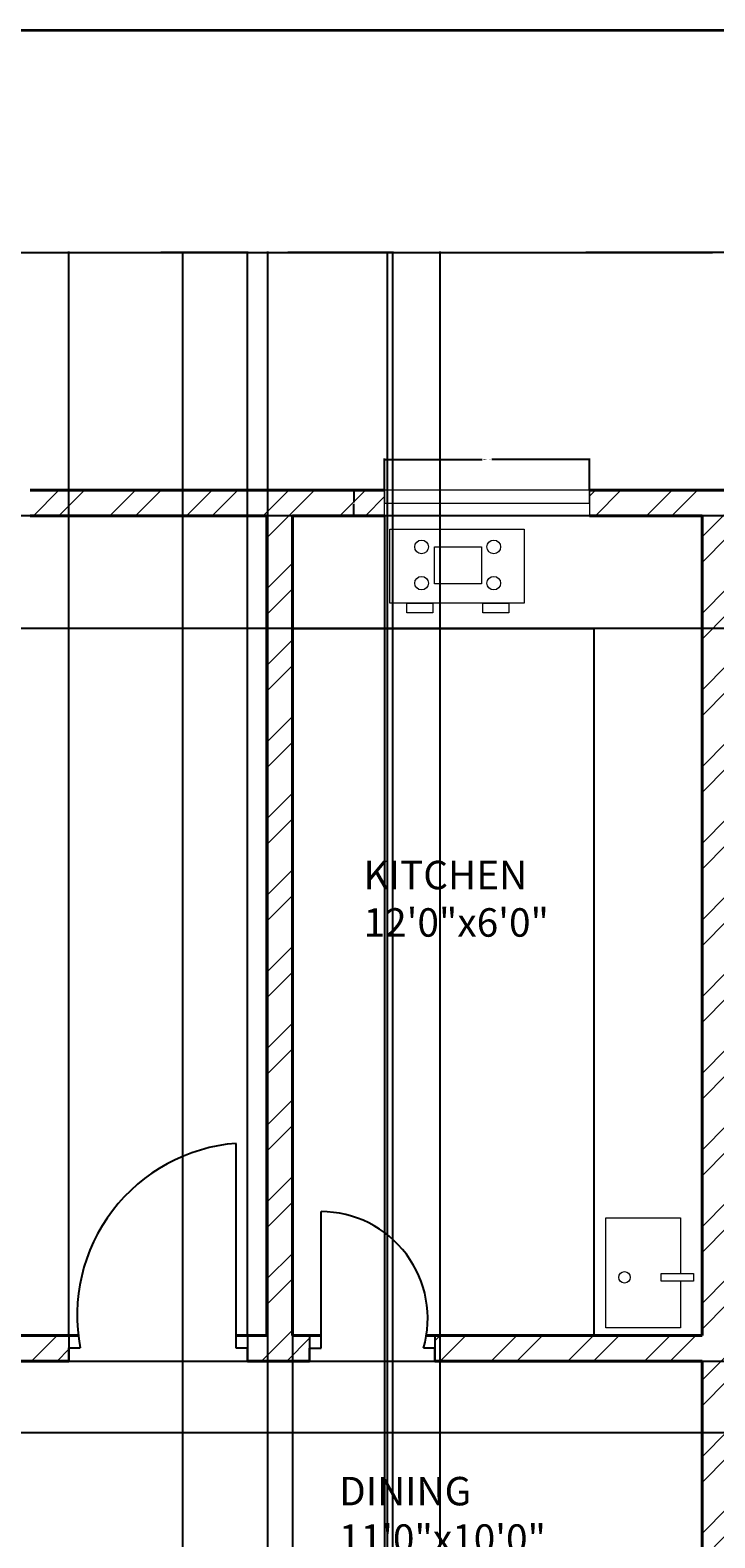
# Model space of a CAD drawing. Units: inches. Extents: x 2063 to 2617, y 1299 to 2210.
# Tile 14 of 22: x 2218 to 2338, y 1945 to 2210. Entities that reach past the tile are written whole.
import ezdxf

# ---------------------------------------------------------------- set-up
doc = ezdxf.new("R2010")
doc.units = ezdxf.units.IN
for name, color, linetype, lineweight in [('A-ANNO-DIMS', 2, 'Continuous', 18), ('A-ANNO-TTLB', 7, 'Continuous', 35), ('A-AREA-IDEN', 7, 'Continuous', 18), ('A-DOOR', 11, 'Continuous', 25), ('A-EQPM', 8, 'Continuous', 18), ('A-FLOR-CASE', 8, 'Continuous', 25), ('A-FLOR-FIXT', 8, 'Continuous', 18), ('A-GLAZ', 123, 'Continuous', 18), ('A-WALL', 7, 'Continuous', 40)]:
    doc.layers.add(name, color=color, linetype=linetype, lineweight=lineweight)
doc.layers.add('A-WALL-PATT', color=215, linetype='Continuous', lineweight=13, true_color=0xa953a0)
doc.styles.get("Standard").update_dxf_attribs({"font": 'arial.ttf'})
doc.dimstyles.get("Standard").update_dxf_attribs({"dimtxt": 0.18, "dimasz": 0.18, "dimexe": 0.18, "dimexo": 0.0625, "dimgap": 0.09, "dimtad": 0, "dimtih": 1, "dimtoh": 1, "dimdec": 4, "dimzin": 0, "dimdsep": 46, "dimtxsty": 'Standard', "dimcen": 0.09, "dimadec": 0, "dimazin": 0, "dimtfac": 1, "dimtdec": 4, "dimtofl": 0, "dimtmove": 0, "dimatfit": 3, "dimfxl": 1, "dimtolj": 1, "dimtzin": 0, "dimarcsym": 0})

# ---------------------------------------------------------------- blocks, each defined once
blk = doc.blocks.new('WIN-36IN')
for p, q in [((0, 0), (0, 4.5)), ((0, 4.5), (0, 2.25)), ((36, 4.5), (0, 4.5)), ((36, 2.25), (36, 4.5)), ((36, 4.5), (36, 0)), ((0, 2.25), (36, 2.25)), ((0, 0), (36, 0))]:
    blk.add_line(p, q)
blk = doc.blocks.new('COOKTOP-4BURNER')
for points in [[(0, 14.7), (23.64, 14.7), (23.64, 1.68), (0, 1.68)], [(7.88, 11.59), (16.13, 11.59), (16.13, 5.1), (7.88, 5.1)], [(3.01, 1.68), (3.01, 1.68), (3.01, 1.68), (3.01, 1.68)], [(3.01, 1.68), (7.59, 1.68), (7.59, 0), (3.01, 0)], [(16.36, 1.68), (20.94, 1.68), (20.94, 0), (16.36, 0)]]:
    blk.add_lwpolyline(points, close=True)
for centre in [(5.6, 11.57), (18.3, 11.57), (5.6, 5.19), (18.3, 5.19)]:
    blk.add_circle(centre, 1.2)
blk = doc.blocks.new('SINK-SINGLE')
blk.add_lwpolyline([(13.12, 8.22), (13.12, 0), (0, 0), (0, 19.36), (13.12, 19.36), (13.12, 9.57)])
blk.add_lwpolyline([(9.77, 9.57), (15.43, 9.57), (15.43, 8.22), (9.77, 8.22)], close=True)
blk.add_circle((3.31, 8.89), 1.01)
blk = doc.blocks.new('*D19')
at = {"layer": 'A-ANNO-DIMS', "color": 0, "lineweight": -2, "transparency": 16777216}
for p, q in [((2280.35, 2128.87), (2280.35, 2134.39)), ((2280.53, 2134.21), (2297.5, 2134.21)), ((2316.17, 2134.21), (2299.19, 2134.21)), ((2316.35, 2128.87), (2316.35, 2134.39))]:
    blk.add_line(p, q, dxfattribs=at)
at = {"layer": 'A-ANNO-DIMS', "color": 0, "transparency": 16777216}
for points in [[(2280.53, 2134.24), (2280.53, 2134.18), (2280.35, 2134.21)], [(2316.17, 2134.24), (2316.17, 2134.18), (2316.35, 2134.21)]]:
    blk.add_solid(points, dxfattribs=at)
at = {"layer": 'Defpoints', "color": 0, "transparency": 16777216}
for p in [(2316.35, 2134.21), (2280.35, 2128.81), (2316.35, 2128.81)]:
    blk.add_point(p, dxfattribs=at)
at = {"layer": 'A-ANNO-DIMS', "color": 0, "transparency": 16777216, "insert": (2298.35, 2134.21), "char_height": 0.18, "attachment_point": 5}
blk.add_mtext('\\A1;WIN. 36 TYP.', dxfattribs=at)
blk = doc.blocks.new('*D20')
at = {"layer": 'A-ANNO-DIMS', "color": 0, "lineweight": -2, "transparency": 16777216}
for p, q in [((2280.29, 2128.81), (2274.77, 2128.81)), ((2274.95, 2128.63), (2274.95, 2126.74)), ((2274.95, 2124.49), (2274.95, 2126.38)), ((2280.29, 2124.31), (2274.77, 2124.31))]:
    blk.add_line(p, q, dxfattribs=at)
at = {"layer": 'A-ANNO-DIMS', "color": 0, "transparency": 16777216}
for points in [[(2274.92, 2128.63), (2274.98, 2128.63), (2274.95, 2128.81)], [(2274.92, 2124.49), (2274.98, 2124.49), (2274.95, 2124.31)]]:
    blk.add_solid(points, dxfattribs=at)
at = {"layer": 'Defpoints', "color": 0, "transparency": 16777216}
for p in [(2274.95, 2128.81), (2280.35, 2128.81), (2280.35, 2124.31)]:
    blk.add_point(p, dxfattribs=at)
at = {"layer": 'A-ANNO-DIMS', "color": 0, "transparency": 16777216, "insert": (2274.95, 2126.56), "char_height": 0.18, "attachment_point": 5}
blk.add_mtext('\\A1;5 TYP.', dxfattribs=at)
blk = doc.blocks.new('*D31')
at = {"layer": 'A-ANNO-DIMS', "color": 0, "lineweight": -2, "transparency": 16777216}
for p, q in [((2123.14, 2128.87), (2123.14, 2170.74)), ((2123.32, 2170.56), (2338, 2170.56)), ((2553.46, 2170.56), (2338.79, 2170.56)), ((2553.64, 2128.87), (2553.64, 2170.74))]:
    blk.add_line(p, q, dxfattribs=at)
at = {"layer": 'A-ANNO-DIMS', "color": 0, "transparency": 16777216}
for points in [[(2123.32, 2170.59), (2123.32, 2170.53), (2123.14, 2170.56)], [(2553.46, 2170.59), (2553.46, 2170.53), (2553.64, 2170.56)]]:
    blk.add_solid(points, dxfattribs=at)
at = {"layer": 'Defpoints', "color": 0, "transparency": 16777216}
for p in [(2553.64, 2170.56), (2123.14, 2128.81), (2553.64, 2128.81)]:
    blk.add_point(p, dxfattribs=at)
at = {"layer": 'A-ANNO-DIMS', "color": 0, "transparency": 16777216, "insert": (2338.39, 2170.56), "char_height": 0.18, "attachment_point": 5}
blk.add_mtext('\\A1;430.5', dxfattribs=at)
blk = doc.blocks.new('*D50')
at = {"layer": 'A-ANNO-DIMS', "color": 0, "lineweight": -2, "transparency": 16777216}
for p, q in [((2264.14, 2124.25), (2264.14, 1317.7)), ((2280.35, 2124.25), (2280.35, 1317.7)), ((2264.32, 1317.88), (2271.79, 1317.88)), ((2280.17, 1317.88), (2272.7, 1317.88))]:
    blk.add_line(p, q, dxfattribs=at)
at = {"layer": 'A-ANNO-DIMS', "color": 0, "transparency": 16777216}
for points in [[(2264.32, 1317.91), (2264.32, 1317.85), (2264.14, 1317.88)], [(2280.17, 1317.91), (2280.17, 1317.85), (2280.35, 1317.88)]]:
    blk.add_solid(points, dxfattribs=at)
at = {"layer": 'Defpoints', "color": 0, "transparency": 16777216}
for p in [(2264.14, 2124.31), (2280.35, 2124.31), (2280.35, 1317.88)]:
    blk.add_point(p, dxfattribs=at)
at = {"layer": 'A-ANNO-DIMS', "color": 0, "transparency": 16777216, "insert": (2272.25, 1317.88), "char_height": 0.18, "attachment_point": 5}
blk.add_mtext('\\A1;16.204', dxfattribs=at)
blk = doc.blocks.new('*D53')
at = {"layer": 'A-ANNO-DIMS', "color": 0, "lineweight": -2, "transparency": 16777216}
for p, q in [((2412.58, 2124.31), (2081.21, 2124.31)), ((2081.39, 2124.13), (2081.39, 2114.6)), ((2081.39, 2104.7), (2081.39, 2114.23)), ((2412.58, 2104.52), (2081.21, 2104.52))]:
    blk.add_line(p, q, dxfattribs=at)
at = {"layer": 'A-ANNO-DIMS', "color": 0, "transparency": 16777216}
for points in [[(2081.36, 2124.13), (2081.42, 2124.13), (2081.39, 2124.31)], [(2081.36, 2104.7), (2081.42, 2104.7), (2081.39, 2104.52)]]:
    blk.add_solid(points, dxfattribs=at)
at = {"layer": 'Defpoints', "color": 0, "transparency": 16777216}
for p in [(2412.64, 2124.31), (2081.39, 2104.52), (2412.64, 2104.52)]:
    blk.add_point(p, dxfattribs=at)
at = {"layer": 'A-ANNO-DIMS', "color": 0, "transparency": 16777216, "insert": (2081.39, 2114.42), "char_height": 0.18, "attachment_point": 5}
blk.add_mtext('\\A1;19.792', dxfattribs=at)
blk = doc.blocks.new('*D59')
at = {"layer": 'A-ANNO-DIMS', "color": 0, "lineweight": -2, "transparency": 16777216}
for p, q in [((2290.14, 1554.56), (2290.14, 2170.74)), ((2290.32, 2170.56), (2315.07, 2170.56)), ((2340.46, 2170.56), (2315.72, 2170.56)), ((2340.64, 1554.56), (2340.64, 2170.74))]:
    blk.add_line(p, q, dxfattribs=at)
at = {"layer": 'A-ANNO-DIMS', "color": 0, "transparency": 16777216}
for points in [[(2290.32, 2170.59), (2290.32, 2170.53), (2290.14, 2170.56)], [(2340.46, 2170.59), (2340.46, 2170.53), (2340.64, 2170.56)]]:
    blk.add_solid(points, dxfattribs=at)
at = {"layer": 'Defpoints', "color": 0, "transparency": 16777216}
for p in [(2340.64, 2170.56), (2290.14, 1554.5), (2340.64, 1554.5)]:
    blk.add_point(p, dxfattribs=at)
at = {"layer": 'A-ANNO-DIMS', "color": 0, "transparency": 16777216, "insert": (2315.39, 2170.56), "char_height": 0.18, "attachment_point": 5}
blk.add_mtext('\\A1;50.5', dxfattribs=at)
blk = doc.blocks.new('*D62')
at = {"layer": 'A-ANNO-DIMS', "color": 0, "lineweight": -2, "transparency": 16777216}
for p, q in [((2259.81, 1437.87), (2259.81, 2170.74)), ((2259.99, 2170.56), (2270.4, 2170.56)), ((2281.61, 2170.56), (2271.19, 2170.56)), ((2281.79, 1437.87), (2281.79, 2170.74))]:
    blk.add_line(p, q, dxfattribs=at)
at = {"layer": 'A-ANNO-DIMS', "color": 0, "transparency": 16777216}
for points in [[(2259.99, 2170.59), (2259.99, 2170.53), (2259.81, 2170.56)], [(2281.61, 2170.59), (2281.61, 2170.53), (2281.79, 2170.56)]]:
    blk.add_solid(points, dxfattribs=at)
at = {"layer": 'Defpoints', "color": 0, "transparency": 16777216}
for p in [(2281.79, 2170.56), (2259.81, 1437.81), (2281.79, 1437.81)]:
    blk.add_point(p, dxfattribs=at)
at = {"layer": 'A-ANNO-DIMS', "color": 0, "transparency": 16777216, "insert": (2270.8, 2170.56), "char_height": 0.18, "attachment_point": 5}
blk.add_mtext('\\A1;21.98', dxfattribs=at)
blk = doc.blocks.new('*D63')
at = {"layer": 'A-ANNO-DIMS', "color": 0, "lineweight": -2, "transparency": 16777216}
for p, q in [((2244.87, 1562.37), (2244.87, 2170.74)), ((2245.05, 2170.56), (2262.4, 2170.56)), ((2280.68, 2170.56), (2263.33, 2170.56)), ((2280.86, 1562.37), (2280.86, 2170.74))]:
    blk.add_line(p, q, dxfattribs=at)
at = {"layer": 'A-ANNO-DIMS', "color": 0, "transparency": 16777216}
for points in [[(2245.05, 2170.59), (2245.05, 2170.53), (2244.87, 2170.56)], [(2280.68, 2170.59), (2280.68, 2170.53), (2280.86, 2170.56)]]:
    blk.add_solid(points, dxfattribs=at)
at = {"layer": 'Defpoints', "color": 0, "transparency": 16777216}
for p in [(2280.86, 2170.56), (2244.87, 1562.31), (2280.86, 1562.31)]:
    blk.add_point(p, dxfattribs=at)
at = {"layer": 'A-ANNO-DIMS', "color": 0, "transparency": 16777216, "insert": (2262.86, 2170.56), "char_height": 0.18, "attachment_point": 5}
blk.add_mtext('\\A1;35.995', dxfattribs=at)
blk = doc.blocks.new('*D64')
at = {"layer": 'A-ANNO-DIMS', "color": 0, "lineweight": -2, "transparency": 16777216}
for p, q in [((2224.84, 1980.37), (2224.84, 2170.74)), ((2225.02, 2170.56), (2240.08, 2170.56)), ((2256.07, 2170.56), (2241.01, 2170.56)), ((2256.25, 1980.37), (2256.25, 2170.74))]:
    blk.add_line(p, q, dxfattribs=at)
at = {"layer": 'A-ANNO-DIMS', "color": 0, "transparency": 16777216}
for points in [[(2225.02, 2170.59), (2225.02, 2170.53), (2224.84, 2170.56)], [(2256.07, 2170.59), (2256.07, 2170.53), (2256.25, 2170.56)]]:
    blk.add_solid(points, dxfattribs=at)
at = {"layer": 'Defpoints', "color": 0, "transparency": 16777216}
for p in [(2256.25, 2170.56), (2224.84, 1980.31), (2256.25, 1980.31)]:
    blk.add_point(p, dxfattribs=at)
at = {"layer": 'A-ANNO-DIMS', "color": 0, "transparency": 16777216, "insert": (2240.54, 2170.56), "char_height": 0.18, "attachment_point": 5}
blk.add_mtext('\\A1;31.413', dxfattribs=at)
blk = doc.blocks.new('*D67')
at = {"layer": 'A-ANNO-DIMS', "color": 0, "lineweight": -2, "transparency": 16777216}
for p, q in [((2127.71, 1975.81), (2595.57, 1975.81)), ((2595.39, 1975.63), (2595.39, 1969.73)), ((2595.39, 1963.46), (2595.39, 1969.36)), ((2128.42, 1963.28), (2595.57, 1963.28))]:
    blk.add_line(p, q, dxfattribs=at)
at = {"layer": 'A-ANNO-DIMS', "color": 0, "transparency": 16777216}
for points in [[(2595.36, 1975.63), (2595.42, 1975.63), (2595.39, 1975.81)], [(2595.36, 1963.46), (2595.42, 1963.46), (2595.39, 1963.28)]]:
    blk.add_solid(points, dxfattribs=at)
at = {"layer": 'Defpoints', "color": 0, "transparency": 16777216}
for p in [(2127.64, 1975.81), (2128.36, 1963.28), (2595.39, 1963.28)]:
    blk.add_point(p, dxfattribs=at)
at = {"layer": 'A-ANNO-DIMS', "color": 0, "transparency": 16777216, "insert": (2595.39, 1969.55), "char_height": 0.18, "attachment_point": 5}
blk.add_mtext('\\A1;12.533', dxfattribs=at)

msp = doc.modelspace()

# ---------------------------------------------------------------- hatches: boundary and pattern name
at = {"layer": 'A-WALL-PATT'}
h = msp.add_hatch(dxfattribs=at)
h.set_pattern_fill('ANSI32', color=256)
h.paths.add_polyline_path([(2127.6442, 2124.3122), (2158.0405, 2124.3122), (2158.0405, 2126.5622), (2158.0405, 2128.8122), (2123.1442, 2128.8122), (2123.1442, 2082.1152), (2127.6442, 2082.1152)])
h.paths.add_polyline_path([(2280.3482, 2128.8122), (2218.0405, 2128.8122), (2218.0405, 2124.3122), (2259.6442, 2124.3122), (2259.6442, 1980.3122), (2256.2494, 1980.3122), (2256.2494, 1975.8122), (2267.1725, 1975.8122), (2267.1725, 1978.0622), (2267.1725, 1980.3122), (2264.1442, 1980.3122), (2264.1442, 2124.3122), (2280.3482, 2124.3122)])
h.paths.add_polyline_path([(2451.1703, 2128.8122), (2394.7501, 2128.8122), (2394.7501, 2124.3122), (2412.6442, 2124.3122), (2412.6442, 1980.3122), (2409.375, 1980.3122), (2409.375, 1975.8122), (2420.2747, 1975.8122), (2420.2747, 1978.0622), (2420.2747, 1980.3122), (2417.1442, 1980.3122), (2417.1442, 2124.3122), (2451.1703, 2124.3122), (2451.1703, 2126.5622)])
h = msp.add_hatch(dxfattribs=at)
h.set_pattern_fill('ANSI32', color=256)
h.paths.add_polyline_path([(2553.6442, 2128.8122), (2511.1703, 2128.8122), (2511.1703, 2124.3122), (2549.1442, 2124.3122), (2549.1442, 2095.662), (2553.6442, 2095.662)])
h.paths.add_polyline_path([(2553.6442, 2035.662), (2549.1442, 2035.662), (2549.1442, 1980.3122), (2503.7214, 1980.3122), (2503.7214, 1975.8122), (2549.1442, 1975.8122), (2549.1442, 1962.9693), (2553.6442, 1962.9693)])
h.paths.add_polyline_path([(2553.6442, 1938.9693), (2549.1442, 1938.9693), (2549.1442, 1927.8122), (2477.1442, 1927.8122), (2477.1442, 1975.8122), (2481.2918, 1975.8122), (2481.2918, 1980.3122), (2453.2648, 1980.3122), (2453.2648, 1975.8122), (2472.6442, 1975.8122), (2472.6442, 1868.3122), (2400.6442, 1868.3122), (2400.6442, 1861.3782), (2405.1442, 1861.3782), (2405.1442, 1863.8122), (2480.9699, 1863.8122), (2480.9699, 1866.0622), (2480.9699, 1868.3122), (2477.1442, 1868.3122), (2477.1442, 1923.3122), (2549.1442, 1923.3122), (2549.1442, 1908.8504), (2553.6442, 1908.8504)])
h.paths.add_polyline_path([(2553.6442, 1884.8504), (2549.1442, 1884.8504), (2549.1442, 1868.3122), (2501.0636, 1868.3122), (2501.0636, 1863.8122), (2549.1442, 1863.8122), (2549.1442, 1826.0298), (2553.6442, 1826.0298)])
h.paths.add_polyline_path([(2388.1504, 1980.3122), (2340.6442, 1980.3122), (2340.6442, 2124.3122), (2358.7501, 2124.3122), (2358.7501, 2128.8122), (2316.3482, 2128.8122), (2316.3482, 2124.3122), (2336.1442, 2124.3122), (2336.1442, 1980.3122), (2289.1737, 1980.3122), (2289.1737, 1975.8122), (2336.1442, 1975.8122), (2336.1442, 1619.3122), (2333.1433, 1619.3122), (2333.1433, 1614.8122), (2344.1671, 1614.8122), (2344.1671, 1617.0622), (2344.1671, 1619.3122), (2340.6442, 1619.3122), (2340.6442, 1975.8122), (2388.1504, 1975.8122), (2388.1504, 1978.0622)])
h.paths.add_polyline_path([(2290.1442, 1614.8122), (2301.4594, 1614.8122), (2301.4594, 1617.0622), (2301.4594, 1619.3122), (2285.6442, 1619.3122), (2285.6442, 1566.8122), (2280.8619, 1566.8122), (2280.8619, 1564.5622), (2280.8619, 1562.3122), (2285.6442, 1562.3122), (2285.6442, 1442.3122), (2281.7879, 1442.3122), (2281.7879, 1437.8122), (2285.6442, 1437.8122), (2285.6442, 1401.8122), (2290.1442, 1401.8122)])
h.paths.add_polyline_path([(2549.1442, 1731.8122), (2405.1442, 1731.8122), (2405.1442, 1834.4638), (2402.8942, 1834.4638), (2400.6442, 1834.4638), (2400.6442, 1727.3122), (2549.1442, 1727.3122)])
h.paths.add_polyline_path([(2553.6442, 1766.0298), (2551.3942, 1766.0298), (2549.1442, 1766.0298), (2549.1442, 1686.7767), (2553.6442, 1686.7767)])
h.paths.add_polyline_path([(2553.6442, 1638.7767), (2551.3942, 1638.7767), (2549.1442, 1638.7767), (2549.1442, 1619.3122), (2448.6442, 1619.3122), (2448.6442, 1610.5671), (2450.8942, 1610.5671), (2453.1442, 1610.5671), (2453.1442, 1614.8122), (2549.1442, 1614.8122), (2549.1442, 1601.6421), (2553.6442, 1601.6421)])
h.paths.add_polyline_path([(2553.6442, 1577.6421), (2551.3942, 1577.6421), (2549.1442, 1577.6421), (2549.1442, 1566.8122), (2453.1442, 1566.8122), (2453.1442, 1591.5045), (2451.0335, 1591.5045), (2448.6442, 1591.5045), (2448.6442, 1566.8122), (2434.0475, 1566.8122), (2434.0475, 1562.3122), (2549.1442, 1562.3122), (2549.1442, 1533.48), (2553.6442, 1533.48)])
h.paths.add_polyline_path([(2553.6442, 1473.48), (2549.1442, 1473.48), (2549.1442, 1442.3122), (2502.6258, 1442.3122), (2502.6258, 1437.8122), (2549.1442, 1437.8122), (2549.1442, 1401.8122), (2553.6442, 1401.8122)])
h.paths.add_polyline_path([(2395.6442, 1562.3122), (2400.0901, 1562.3122), (2400.0901, 1564.5622), (2400.0901, 1566.8122), (2395.6442, 1566.8122), (2395.6442, 1619.3122), (2379.1127, 1619.3122), (2379.1127, 1614.8122), (2391.1442, 1614.8122), (2391.1442, 1401.8122), (2395.6442, 1401.8122), (2395.6442, 1437.8122), (2399.2425, 1437.8122), (2399.2425, 1440.0622), (2399.2425, 1442.3122), (2395.6442, 1442.3122)])
h.paths.add_polyline_path([(2442.6258, 1442.3122), (2419.6262, 1442.3122), (2419.6262, 1437.8122), (2442.6258, 1437.8122), (2442.6258, 1440.0622)])
h.paths.add_polyline_path([(2127.6442, 1480.2532), (2125.3942, 1480.2532), (2123.1442, 1480.2532), (2123.1442, 1401.8122), (2127.6442, 1401.8122), (2127.6442, 1437.8122), (2145.1538, 1437.8122), (2145.1538, 1440.0622), (2145.1538, 1442.3122), (2127.6442, 1442.3122)])
h.paths.add_polyline_path([(2259.809, 1442.3122), (2205.1538, 1442.3122), (2205.1538, 1437.8122), (2259.809, 1437.8122), (2259.809, 1440.0622)])
h.paths.add_polyline_path([(2127.6442, 1659.7652), (2123.1442, 1659.7652), (2123.1442, 1605.5161), (2125.3942, 1605.5161), (2127.6442, 1605.5161), (2127.6442, 1614.8122), (2223.6442, 1614.8122), (2223.6442, 1611.2723), (2228.1442, 1611.2723), (2228.1442, 1619.3122), (2127.6442, 1619.3122)])
h.paths.add_polyline_path([(2244.8673, 1566.8122), (2228.1442, 1566.8122), (2228.1442, 1590.8122), (2225.8942, 1590.8122), (2223.6442, 1590.8122), (2223.6442, 1566.8122), (2127.6442, 1566.8122), (2127.6442, 1581.5161), (2123.1442, 1581.5161), (2123.1442, 1540.2532), (2127.6442, 1540.2532), (2127.6442, 1562.3122), (2244.8673, 1562.3122), (2244.8673, 1564.5622)])
h.paths.add_polyline_path([(2172.5174, 1868.3122), (2127.6442, 1868.3122), (2127.6442, 1886.5833), (2123.1442, 1886.5833), (2123.1442, 1832.6633), (2127.6442, 1832.6633), (2127.6442, 1863.8122), (2172.5174, 1863.8122), (2172.5174, 1866.0622)])
h.paths.add_polyline_path([(2276.1442, 1868.3122), (2204.1442, 1868.3122), (2204.1442, 1923.3122), (2204.1442, 1975.8122), (2224.8362, 1975.8122), (2224.8362, 1978.1097), (2224.8362, 1980.3122), (2195.0729, 1980.3122), (2195.0729, 1978.0622), (2195.0729, 1975.8122), (2199.6442, 1975.8122), (2199.6442, 1927.8122), (2127.6442, 1927.8122), (2127.6442, 1942.3492), (2123.1442, 1942.3492), (2123.1442, 1910.5833), (2127.6442, 1910.5833), (2127.6442, 1923.3122), (2199.6442, 1923.3122), (2199.6442, 1868.3122), (2194.8228, 1868.3122), (2194.8228, 1864.7337), (2194.8228, 1863.8122), (2271.6442, 1863.8122), (2271.6442, 1860.0507), (2276.1442, 1860.0507)])
h.paths.add_polyline_path([(2276.1442, 1829.994), (2273.8942, 1829.994), (2271.6442, 1829.994), (2271.6442, 1731.8122), (2127.6442, 1731.8122), (2127.6442, 1772.6633), (2123.1442, 1772.6633), (2123.1442, 1707.7652), (2127.6442, 1707.7652), (2127.6442, 1727.3122), (2276.1442, 1727.3122)])
h.paths.add_polyline_path([(2127.6442, 2022.1152), (2123.1442, 2022.1152), (2123.1442, 1966.3492), (2127.6442, 1966.3492), (2127.6442, 1975.8122), (2174.2082, 1975.8122), (2174.2082, 1978.0622), (2174.2082, 1980.3122), (2127.6442, 1980.3122)])
h.paths.add_polyline_path([(2361.9755, 1678.588), (2398.4558, 1678.588), (2398.4558, 1697.2453), (2361.9755, 1697.2453)], flags=9)
h.paths.add_polyline_path([(2351.5397, 1780.4072), (2386.1987, 1780.4072), (2386.1987, 1790.7107), (2351.5397, 1790.7107)], flags=25)
h.paths.add_polyline_path([(2350.6753, 1940.9321), (2387.6024, 1940.9321), (2387.6024, 1959.5894), (2350.6753, 1959.5894)], flags=25)
h.paths.add_polyline_path([(2254.9545, 1684.638), (2295.0943, 1684.638), (2295.0943, 1703.2953), (2254.9545, 1703.2953)], flags=9)
h.paths.add_polyline_path([(2282.4946, 1782.4438), (2317.1535, 1782.4438), (2317.1535, 1792.7474), (2282.4946, 1792.7474)], flags=9)
h.paths.add_polyline_path([(2270.327, 1939.2854), (2307.254, 1939.2854), (2307.254, 1957.9428), (2270.327, 1957.9428)], flags=9)

# ---------------------------------------------------------------- linework, layer by layer
at = {"layer": 'A-ANNO-TTLB'}
msp.add_lwpolyline([(2062.5792, 2209.6485), (2617.0648, 2209.6485), (2617.0648, 1299.1125), (2062.5792, 1299.1125)], close=True, dxfattribs=at)
at = {"layer": 'A-DOOR'}
for p, q in [((2254.2494, 1978.0622), (2254.2494, 2014.0622)), ((2269.1725, 1978.0622), (2269.1725, 2002.0622)), ((2224.8362, 1980.3122), (2224.8362, 1976.9314)), ((2256.2494, 1980.3122), (2256.2494, 1980.3122)), ((2256.2494, 1980.3122), (2256.2494, 1975.8122)), ((2267.1725, 1980.3122), (2267.1725, 1975.8122)), ((2289.1737, 1980.3122), (2289.1737, 1975.8122)), ((2224.8362, 1975.8122), (2224.8362, 1978.1097)), ((2224.8362, 1978.1097), (2226.8362, 1978.1097)), ((2224.8362, 1976.9314), (2224.8362, 1975.8122)), ((2256.2494, 1978.0622), (2254.2494, 1978.0622)), ((2256.2494, 1975.8122), (2256.2494, 1978.0622)), ((2267.1725, 1975.8122), (2267.1725, 1978.0622)), ((2267.1725, 1978.0622), (2269.1725, 1978.0622)), ((2289.1737, 1978.0622), (2287.1737, 1978.0622)), ((2289.1737, 1975.8122), (2289.1737, 1978.0622))]:
    msp.add_line(p, q, dxfattribs=at)
for centre, radius, start, end in [((2256.6211, 1983.8265), 30.3285, 94.485092, 190.865083), ((2269.1725, 1983.3113), 18.7509, 343.7434, 90)]:
    msp.add_arc(centre, radius, start, end, dxfattribs=at)
at = {"layer": 'A-FLOR-CASE'}
for p, q in [((2264.1442, 2104.5201), (2317.1222, 2104.5201)), ((2317.1222, 2104.5201), (2317.1222, 1980.3122))]:
    msp.add_line(p, q, dxfattribs=at)
at = {"layer": 'A-GLAZ'}
msp.add_line((2280.3482, 2128.8122), (2280.3482, 2128.8122), dxfattribs=at)
at = {"layer": 'A-WALL'}
for p, q in [((2218.0405, 2128.8122), (2280.3482, 2128.8122)), ((2218.0405, 2128.8122), (2280.3482, 2128.8122)), ((2316.3482, 2128.8122), (2358.7501, 2128.8122)), ((2316.3482, 2128.8122), (2358.7501, 2128.8122)), ((2218.0405, 2124.3122), (2259.6442, 2124.3122)), ((2259.6442, 2124.3122), (2259.6442, 1980.3122)), ((2264.1442, 2124.3122), (2264.1442, 1980.3122)), ((2264.1442, 2124.3122), (2280.3482, 2124.3122)), ((2316.3482, 2124.3122), (2336.1442, 2124.3122)), ((2336.1442, 2124.3122), (2336.1442, 1980.3122)), ((2195.0729, 1980.3122), (2226.4969, 1980.3122)), ((2254.2494, 1980.3122), (2259.6442, 1980.3122)), ((2264.1442, 1980.3122), (2269.1725, 1980.3122)), ((2287.682, 1980.3122), (2336.1442, 1980.3122)), ((2204.1442, 1975.8122), (2224.8362, 1975.8122)), ((2256.2494, 1975.8122), (2267.1725, 1975.8122)), ((2289.1737, 1975.8122), (2336.1442, 1975.8122)), ((2336.1442, 1975.8122), (2336.1442, 1619.3122))]:
    msp.add_line(p, q, dxfattribs=at)

# ---------------------------------------------------------------- block references
at = {"layer": 'A-EQPM'}
msp.add_blockref('COOKTOP-4BURNER', (2281.237, 2107.294), dxfattribs=at)
at = {"layer": 'A-FLOR-FIXT'}
msp.add_blockref('SINK-SINGLE', (2319.213, 1981.624), dxfattribs=at)
at = {"layer": 'A-GLAZ'}
msp.add_blockref('WIN-36IN', (2280.348, 2124.312), dxfattribs=at)

# ---------------------------------------------------------------- texts
at = {"layer": 'A-AREA-IDEN', "char_height": 5, "attachment_point": 1}
for s, width, insert in [('KITCHEN\\P12\'0"x6\'0"', 78.230121, (2276.6461, 2063.7058)), ('DINING\\P11\'0"x10\'0"  ', 126.60671, (2272.3376, 1955.4547))]:
    msp.add_mtext_dynamic_manual_height_columns(s, width=width, gutter_width=12.5, heights=[0], dxfattribs=dict(at, insert=insert))

# ---------------------------------------------------------------- dimensions: what is measured, and where the dimension line sits
at = {"layer": 'A-ANNO-DIMS'}
for base, p1, p2, override, picture, middle in [((2553.6442, 2170.5622), (2123.1442, 2128.8122), (2553.6442, 2128.8122), {"dimdec": 1, "dimlfac": 1, "dimrnd": 0, "dimzin": 0, "dimdsep": 46, "dimlunit": 2}, '*D31', (2338.3942, 2170.5622)), ((2256.2494, 2170.5622), (2224.8362, 1980.3122), (2256.2494, 1980.3122), {"dimdec": 3, "dimlfac": 1, "dimrnd": 0, "dimzin": 0, "dimdsep": 46, "dimlunit": 2}, '*D64', (2240.5428, 2170.5622)), ((2280.8619, 2170.5622), (2244.8673, 1562.3122), (2280.8619, 1562.3122), {"dimdec": 3, "dimlfac": 1, "dimrnd": 0, "dimzin": 0, "dimdsep": 46, "dimlunit": 2}, '*D63', (2262.8646, 2170.5622)), ((2281.7879, 2170.5622), (2259.809, 1437.8122), (2281.7879, 1437.8122), {"dimdec": 2, "dimlfac": 1, "dimrnd": 0, "dimzin": 0, "dimdsep": 46, "dimlunit": 2}, '*D62', (2270.7984, 2170.5622)), ((2340.6442, 2170.5622), (2290.1442, 1554.4994), (2340.6442, 1554.4994), {"dimdec": 1, "dimlfac": 1, "dimrnd": 0, "dimzin": 0, "dimdsep": 46, "dimlunit": 2}, '*D59', (2315.3942, 2170.5622)), ((2280.3482, 1317.8821), (2264.1442, 2124.3122), (2280.3482, 2124.3122), {"dimdec": 3, "dimlfac": 1, "dimrnd": 0, "dimzin": 0, "dimdsep": 46, "dimlunit": 2}, '*D50', (2272.2462, 1317.8821))]:
    dim = msp.add_linear_dim(base=base, p1=p1, p2=p2, dimstyle='Standard', override=override, dxfattribs=at)
    dim.commit()
    dim.dimension.update_dxf_attribs({"geometry": picture, "text_midpoint": middle})
dim = msp.add_linear_dim(base=(2316.3482, 2134.2122), p1=(2280.3482, 2128.8122), p2=(2316.3482, 2128.8122), text='WIN. <> TYP.', dimstyle='Standard', override={"dimdec": 0, "dimlfac": 1, "dimrnd": 0, "dimzin": 0, "dimdsep": 46, "dimlunit": 2}, dxfattribs=at)
dim.commit()
dim.dimension.update_dxf_attribs({"geometry": '*D19', "text_midpoint": (2298.3482, 2134.2122)})
dim = msp.add_linear_dim(base=(2274.9482303118, 2128.8121834776), p1=(2280.3482303118, 2124.3121834776), p2=(2280.3482303118, 2128.8121834776), angle=90, text='<> TYP.', dimstyle='Standard', override={"dimdec": 0, "dimlfac": 1, "dimrnd": 0, "dimzin": 0, "dimdsep": 46, "dimlunit": 2}, dxfattribs=at)
dim.commit()
dim.dimension.update_dxf_attribs({"geometry": '*D20', "text_midpoint": (2274.9482303118, 2126.5621834776)})
for base, p1, p2, picture, middle in [((2081.3943, 2104.5201), (2412.6442, 2124.3122), (2412.6442, 2104.5201), '*D53', (2081.3943, 2114.4162)), ((2595.3943, 1963.2791), (2127.6442, 1975.8122), (2128.3589, 1963.2791), '*D67', (2595.3943, 1969.5457))]:
    dim = msp.add_linear_dim(base=base, p1=p1, p2=p2, angle=90, dimstyle='Standard', override={"dimdec": 3, "dimlfac": 1, "dimrnd": 0, "dimzin": 0, "dimdsep": 46, "dimlunit": 2}, dxfattribs=at)
    dim.commit()
    dim.dimension.update_dxf_attribs({"geometry": picture, "text_midpoint": middle})

doc.saveas('drawing.dxf')
